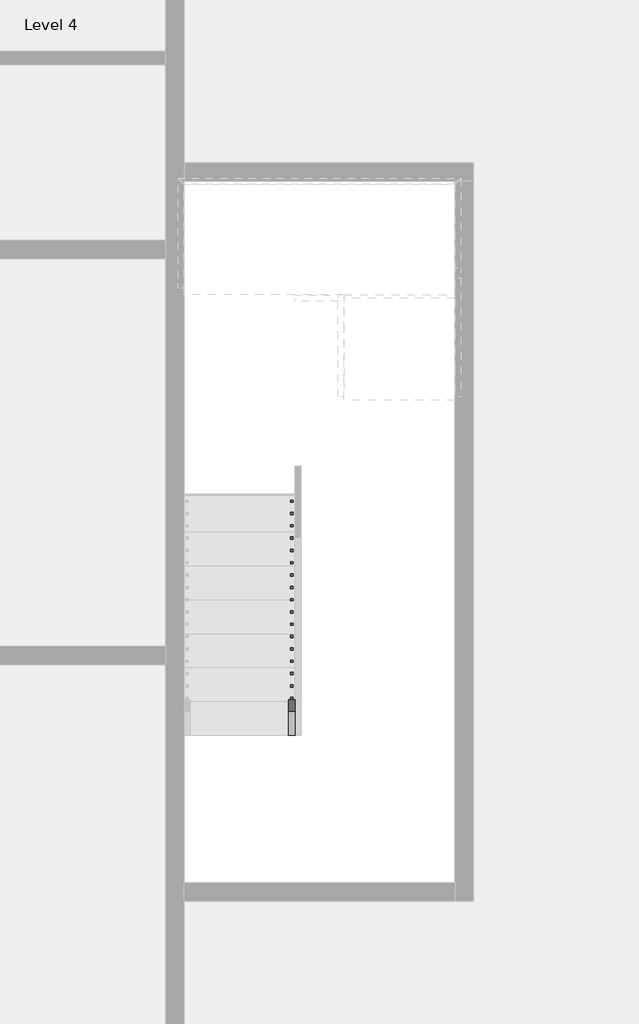
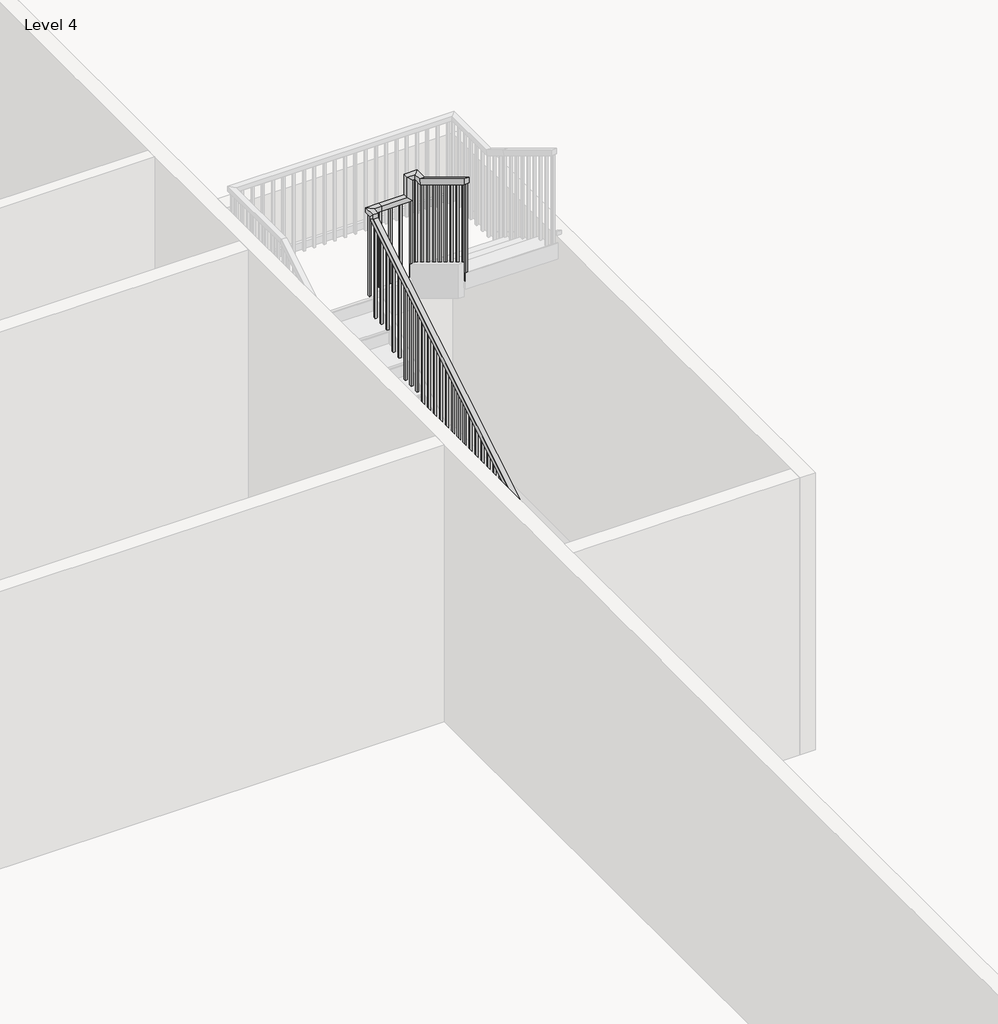
# One storey, part 5 of 8: 1 railing.
"""IFC4 building model written with IfcOpenShell, lengths in millimetres."""

from ifc_helpers import new_model, si_unit, frame, origin, place, context, project, spatial, polyline, outline, extrude, faceted_brep, element, save

model = new_model("IFC4")

# Units and contexts
model_context = context("Model", 3, world=origin())
ifc_project = project(units=[si_unit("LENGTHUNIT", "METRE", prefix="MILLI")], contexts=[model_context])

# Site, building, storey
site = spatial("IfcSite", under=ifc_project)
building = spatial("IfcBuilding", under=site)
storey = spatial("IfcBuildingStorey", under=building, Name="Level 4", Elevation=34378.6172466)

# Railing
placement = place(None, origin())
element("IfcRailing", 1, ObjectType="Handrail - Rectangular", at=placement, inside=storey, context=model_context, shape_type="SolidModel", body=[
    faceted_brep([(-2753.8415084, -23154.3851539, 35462.3505799), (-2753.8415084, -23154.3851539, 35402.9491197), (-2703.0415084, -23154.3851539, 35402.9491197), (-2703.0415084, -23154.3851539, 35462.3505799), (-2753.8415084, -19598.3851539, 37617.5020951), (-2753.8415084, -19547.5851539, 37588.8885136), (-2703.0415084, -19547.5851539, 37588.8885136), (-2703.0415084, -19598.3851539, 37617.5020951), (-2753.8415084, -19598.3851539, 37663.6839133), (-2753.8415084, -19547.5851539, 37612.8839133), (-2703.0415084, -19547.5851539, 37612.8839133), (-2703.0415084, -19598.3851539, 37663.6839133), (-2753.8415084, -19471.3851539, 37663.6839133), (-2753.8415084, -19471.3851539, 37612.8839133), (-2703.0415084, -19522.1851539, 37612.8839133), (-2703.0415084, -19522.1851539, 37663.6839133), (-2626.8415084, -19471.3851539, 37663.6839133), (-2626.8415084, -19471.3851539, 37612.8839133), (-2626.8415084, -19522.1851539, 37612.8839133), (-2626.8415084, -19522.1851539, 37663.6839133), (-2372.8415084, -19471.3851539, 37663.6839133), (-2322.0415084, -19471.3851539, 37612.8839133), (-2322.0415084, -19522.1851539, 37612.8839133), (-2372.8415084, -19522.1851539, 37663.6839133), (-2372.8415084, -19471.3851539, 37879.1990648), (-2322.0415084, -19471.3851539, 37828.3990648), (-2322.0415084, -19522.1851539, 37828.3990648), (-2372.8415084, -19522.1851539, 37879.1990648), (-2245.8415084, -19471.3851539, 37879.1990648), (-2245.8415084, -19471.3851539, 37828.3990648), (-2296.6415084, -19522.1851539, 37828.3990648), (-2296.6415084, -19522.1851539, 37879.1990648), (-2245.8415084, -19598.3851539, 37879.1990648), (-2245.8415084, -19612.5775633, 37828.3990648), (-2296.6415084, -19612.5775633, 37828.3990648), (-2296.6415084, -19598.3851539, 37879.1990648), (-2245.8415084, -20360.3851539, 38341.0172466), (-2296.6415084, -20360.3851539, 38341.0172466), (-2296.6415084, -20360.3851539, 38281.6157863), (-2245.8415084, -20360.3851539, 38281.6157863)], [[[0, 1, 2, 3]], [[1, 0, 4, 5]], [[2, 1, 5, 6]], [[3, 2, 6, 7]], [[0, 3, 7, 4]], [[5, 4, 8, 9]], [[6, 5, 9, 10]], [[7, 6, 10, 11]], [[4, 7, 11, 8]], [[9, 8, 12, 13]], [[10, 9, 13, 14]], [[11, 10, 14, 15]], [[8, 11, 15, 12]], [[13, 12, 16, 17]], [[14, 13, 17, 18]], [[15, 14, 18, 19]], [[12, 15, 19, 16]], [[17, 16, 20, 21]], [[18, 17, 21, 22]], [[19, 18, 22, 23]], [[16, 19, 23, 20]], [[21, 20, 24, 25]], [[22, 21, 25, 26]], [[23, 22, 26, 27]], [[20, 23, 27, 24]], [[25, 24, 28, 29]], [[26, 25, 29, 30]], [[27, 26, 30, 31]], [[24, 27, 31, 28]], [[29, 28, 32, 33]], [[30, 29, 33, 34]], [[31, 30, 34, 35]], [[28, 31, 35, 32]], [[36, 37, 38, 39]], [[33, 32, 36, 39]], [[34, 33, 39, 38]], [[35, 34, 38, 37]], [[32, 35, 37, 36]]]),
    extrude(outline(polyline([(-20319.1101539, 38256.6006348), (-20300.0601539, 38245.0551803), (-20300.0601539, 37257.2839133), (-20319.1101539, 37257.2839133), (-20319.1101539, 38256.6006348)])), frame((-2280.7665084, 0.0, 0.0), z_axis=(1.0, 0.0, 0.0), x_axis=(0.0, 1.0, 0.0)), (0.0, 0.0, 1.0), 19.05),
    extrude(outline(polyline([(-20217.5101539, 38195.0248773), (-20198.4601539, 38183.4794227), (-20198.4601539, 37257.2839133), (-20217.5101539, 37257.2839133), (-20217.5101539, 38195.0248773)])), frame((-2280.7665084, 0.0, 0.0), z_axis=(1.0, 0.0, 0.0), x_axis=(0.0, 1.0, 0.0)), (0.0, 0.0, 1.0), 19.05),
    extrude(outline(polyline([(-20115.9101539, 38133.4491197), (-20096.8601539, 38121.9036651), (-20096.8601539, 37257.2839133), (-20115.9101539, 37257.2839133), (-20115.9101539, 38133.4491197)])), frame((-2280.7665084, 0.0, 0.0), z_axis=(1.0, 0.0, 0.0), x_axis=(0.0, 1.0, 0.0)), (0.0, 0.0, 1.0), 19.05),
    extrude(outline(polyline([(-20014.3101539, 38071.8733621), (-19995.2601539, 38060.3279076), (-19995.2601539, 37087.9505799), (-20014.3101539, 37087.9505799), (-20014.3101539, 38071.8733621)])), frame((-2280.7665084, 0.0, 0.0), z_axis=(1.0, 0.0, 0.0), x_axis=(0.0, 1.0, 0.0)), (0.0, 0.0, 1.0), 19.05),
    extrude(outline(polyline([(-19912.7101539, 38010.2976045), (-19893.6601539, 37998.75215), (-19893.6601539, 37087.9505799), (-19912.7101539, 37087.9505799), (-19912.7101539, 38010.2976045)])), frame((-2280.7665084, 0.0, 0.0), z_axis=(1.0, 0.0, 0.0), x_axis=(0.0, 1.0, 0.0)), (0.0, 0.0, 1.0), 19.05),
    extrude(outline(polyline([(-19811.1101539, 37948.721847), (-19792.0601539, 37937.1763924), (-19792.0601539, 37087.9505799), (-19811.1101539, 37087.9505799), (-19811.1101539, 37948.721847)])), frame((-2280.7665084, 0.0, 0.0), z_axis=(1.0, 0.0, 0.0), x_axis=(0.0, 1.0, 0.0)), (0.0, 0.0, 1.0), 19.05),
    extrude(outline(polyline([(-19709.5101539, 37887.1460894), (-19690.4601539, 37875.6006348), (-19690.4601539, 36918.6172466), (-19709.5101539, 36918.6172466), (-19709.5101539, 37887.1460894)])), frame((-2280.7665084, 0.0, 0.0), z_axis=(1.0, 0.0, 0.0), x_axis=(0.0, 1.0, 0.0)), (0.0, 0.0, 1.0), 19.05),
    extrude(outline(polyline([(-19607.9101539, 37825.5703318), (-19588.8601539, 37814.0248773), (-19588.8601539, 36918.6172466), (-19607.9101539, 36918.6172466), (-19607.9101539, 37825.5703318)])), frame((-2280.7665084, 0.0, 0.0), z_axis=(1.0, 0.0, 0.0), x_axis=(0.0, 1.0, 0.0)), (0.0, 0.0, 1.0), 19.05),
    extrude(outline(polyline([(-2331.5665084, -19506.3101539), (-2331.5665084, -19487.2601539), (-2312.5165084, -19487.2601539), (-2312.5165084, -19506.3101539), (-2331.5665084, -19506.3101539)])), frame((0.0, 0.0, 36749.2839133), z_axis=(0.0, 0.0, 1.0), x_axis=(1.0, 0.0, 0.0)), (0.0, 0.0, 1.0), 1079.1151515),
    extrude(outline(polyline([(-2433.1665084, -19506.3101539), (-2433.1665084, -19487.2601539), (-2414.1165084, -19487.2601539), (-2414.1165084, -19506.3101539), (-2433.1665084, -19506.3101539)])), frame((0.0, 0.0, 36749.2839133), z_axis=(0.0, 0.0, 1.0), x_axis=(1.0, 0.0, 0.0)), (0.0, 0.0, 1.0), 863.6),
    extrude(outline(polyline([(-2534.7665084, -19506.3101539), (-2534.7665084, -19487.2601539), (-2515.7165084, -19487.2601539), (-2515.7165084, -19506.3101539), (-2534.7665084, -19506.3101539)])), frame((0.0, 0.0, 36749.2839133), z_axis=(0.0, 0.0, 1.0), x_axis=(1.0, 0.0, 0.0)), (0.0, 0.0, 1.0), 863.6),
    extrude(outline(polyline([(-2636.3665084, -19506.3101539), (-2636.3665084, -19487.2601539), (-2617.3165084, -19487.2601539), (-2617.3165084, -19506.3101539), (-2636.3665084, -19506.3101539)])), frame((0.0, 0.0, 36749.2839133), z_axis=(0.0, 0.0, 1.0), x_axis=(1.0, 0.0, 0.0)), (0.0, 0.0, 1.0), 863.6),
    extrude(outline(polyline([(-19607.9101539, 37552.3279076), (-19588.8601539, 37563.8733621), (-19588.8601539, 36579.9505799), (-19607.9101539, 36579.9505799), (-19607.9101539, 37552.3279076)])), frame((-2737.9665084, 0.0, 0.0), z_axis=(1.0, 0.0, 0.0), x_axis=(0.0, 1.0, 0.0)), (0.0, 0.0, 1.0), 19.05),
    extrude(outline(polyline([(-19709.5101539, 37490.75215), (-19690.4601539, 37502.2976045), (-19690.4601539, 36579.9505799), (-19709.5101539, 36579.9505799), (-19709.5101539, 37490.75215)])), frame((-2737.9665084, 0.0, 0.0), z_axis=(1.0, 0.0, 0.0), x_axis=(0.0, 1.0, 0.0)), (0.0, 0.0, 1.0), 19.05),
    extrude(outline(polyline([(-19811.1101539, 37429.1763924), (-19792.0601539, 37440.721847), (-19792.0601539, 36579.9505799), (-19811.1101539, 36579.9505799), (-19811.1101539, 37429.1763924)])), frame((-2737.9665084, 0.0, 0.0), z_axis=(1.0, 0.0, 0.0), x_axis=(0.0, 1.0, 0.0)), (0.0, 0.0, 1.0), 19.05),
    extrude(outline(polyline([(-19912.7101539, 37367.6006348), (-19893.6601539, 37379.1460894), (-19893.6601539, 36410.6172466), (-19912.7101539, 36410.6172466), (-19912.7101539, 37367.6006348)])), frame((-2737.9665084, 0.0, 0.0), z_axis=(1.0, 0.0, 0.0), x_axis=(0.0, 1.0, 0.0)), (0.0, 0.0, 1.0), 19.05),
    extrude(outline(polyline([(-20014.3101539, 37306.0248773), (-19995.2601539, 37317.5703318), (-19995.2601539, 36410.6172466), (-20014.3101539, 36410.6172466), (-20014.3101539, 37306.0248773)])), frame((-2737.9665084, 0.0, 0.0), z_axis=(1.0, 0.0, 0.0), x_axis=(0.0, 1.0, 0.0)), (0.0, 0.0, 1.0), 19.05),
    extrude(outline(polyline([(-20115.9101539, 37244.4491197), (-20096.8601539, 37255.9945742), (-20096.8601539, 36241.2839133), (-20115.9101539, 36241.2839133), (-20115.9101539, 37244.4491197)])), frame((-2737.9665084, 0.0, 0.0), z_axis=(1.0, 0.0, 0.0), x_axis=(0.0, 1.0, 0.0)), (0.0, 0.0, 1.0), 19.05),
    extrude(outline(polyline([(-20217.5101539, 37182.8733621), (-20198.4601539, 37194.4188166), (-20198.4601539, 36241.2839133), (-20217.5101539, 36241.2839133), (-20217.5101539, 37182.8733621)])), frame((-2737.9665084, 0.0, 0.0), z_axis=(1.0, 0.0, 0.0), x_axis=(0.0, 1.0, 0.0)), (0.0, 0.0, 1.0), 19.05),
    extrude(outline(polyline([(-20319.1101539, 37121.2976045), (-20300.0601539, 37132.8430591), (-20300.0601539, 36241.2839133), (-20319.1101539, 36241.2839133), (-20319.1101539, 37121.2976045)])), frame((-2737.9665084, 0.0, 0.0), z_axis=(1.0, 0.0, 0.0), x_axis=(0.0, 1.0, 0.0)), (0.0, 0.0, 1.0), 19.05),
    extrude(outline(polyline([(-20420.7101539, 37059.721847), (-20401.6601539, 37071.2673015), (-20401.6601539, 36071.9505799), (-20420.7101539, 36071.9505799), (-20420.7101539, 37059.721847)])), frame((-2737.9665084, 0.0, 0.0), z_axis=(1.0, 0.0, 0.0), x_axis=(0.0, 1.0, 0.0)), (0.0, 0.0, 1.0), 19.05),
    extrude(outline(polyline([(-20522.3101539, 36998.1460894), (-20503.2601539, 37009.6915439), (-20503.2601539, 36071.9505799), (-20522.3101539, 36071.9505799), (-20522.3101539, 36998.1460894)])), frame((-2737.9665084, 0.0, 0.0), z_axis=(1.0, 0.0, 0.0), x_axis=(0.0, 1.0, 0.0)), (0.0, 0.0, 1.0), 19.05),
    extrude(outline(polyline([(-20623.9101539, 36936.5703318), (-20604.8601539, 36948.1157863), (-20604.8601539, 36071.9505799), (-20623.9101539, 36071.9505799), (-20623.9101539, 36936.5703318)])), frame((-2737.9665084, 0.0, 0.0), z_axis=(1.0, 0.0, 0.0), x_axis=(0.0, 1.0, 0.0)), (0.0, 0.0, 1.0), 19.05),
    extrude(outline(polyline([(-20725.5101539, 36874.9945742), (-20706.4601539, 36886.5400288), (-20706.4601539, 35902.6172466), (-20725.5101539, 35902.6172466), (-20725.5101539, 36874.9945742)])), frame((-2737.9665084, 0.0, 0.0), z_axis=(1.0, 0.0, 0.0), x_axis=(0.0, 1.0, 0.0)), (0.0, 0.0, 1.0), 19.05),
    extrude(outline(polyline([(-20827.1101539, 36813.4188166), (-20808.0601539, 36824.9642712), (-20808.0601539, 35902.6172466), (-20827.1101539, 35902.6172466), (-20827.1101539, 36813.4188166)])), frame((-2737.9665084, 0.0, 0.0), z_axis=(1.0, 0.0, 0.0), x_axis=(0.0, 1.0, 0.0)), (0.0, 0.0, 1.0), 19.05),
    extrude(outline(polyline([(-20928.7101539, 36751.8430591), (-20909.6601539, 36763.3885136), (-20909.6601539, 35902.6172466), (-20928.7101539, 35902.6172466), (-20928.7101539, 36751.8430591)])), frame((-2737.9665084, 0.0, 0.0), z_axis=(1.0, 0.0, 0.0), x_axis=(0.0, 1.0, 0.0)), (0.0, 0.0, 1.0), 19.05),
    extrude(outline(polyline([(-21030.3101539, 36690.2673015), (-21011.2601539, 36701.812756), (-21011.2601539, 35733.2839133), (-21030.3101539, 35733.2839133), (-21030.3101539, 36690.2673015)])), frame((-2737.9665084, 0.0, 0.0), z_axis=(1.0, 0.0, 0.0), x_axis=(0.0, 1.0, 0.0)), (0.0, 0.0, 1.0), 19.05),
    extrude(outline(polyline([(-21131.9101539, 36628.6915439), (-21112.8601539, 36640.2369985), (-21112.8601539, 35733.2839133), (-21131.9101539, 35733.2839133), (-21131.9101539, 36628.6915439)])), frame((-2737.9665084, 0.0, 0.0), z_axis=(1.0, 0.0, 0.0), x_axis=(0.0, 1.0, 0.0)), (0.0, 0.0, 1.0), 19.05),
    extrude(outline(polyline([(-21233.5101539, 36567.1157863), (-21214.4601539, 36578.6612409), (-21214.4601539, 35563.9505799), (-21233.5101539, 35563.9505799), (-21233.5101539, 36567.1157863)])), frame((-2737.9665084, 0.0, 0.0), z_axis=(1.0, 0.0, 0.0), x_axis=(0.0, 1.0, 0.0)), (0.0, 0.0, 1.0), 19.05),
    extrude(outline(polyline([(-21335.1101539, 36505.5400288), (-21316.0601539, 36517.0854833), (-21316.0601539, 35563.9505799), (-21335.1101539, 35563.9505799), (-21335.1101539, 36505.5400288)])), frame((-2737.9665084, 0.0, 0.0), z_axis=(1.0, 0.0, 0.0), x_axis=(0.0, 1.0, 0.0)), (0.0, 0.0, 1.0), 19.05),
    extrude(outline(polyline([(-21436.7101539, 36443.9642712), (-21417.6601539, 36455.5097257), (-21417.6601539, 35563.9505799), (-21436.7101539, 35563.9505799), (-21436.7101539, 36443.9642712)])), frame((-2737.9665084, 0.0, 0.0), z_axis=(1.0, 0.0, 0.0), x_axis=(0.0, 1.0, 0.0)), (0.0, 0.0, 1.0), 19.05),
    extrude(outline(polyline([(-21538.3101539, 36382.3885136), (-21519.2601539, 36393.9339682), (-21519.2601539, 35394.6172466), (-21538.3101539, 35394.6172466), (-21538.3101539, 36382.3885136)])), frame((-2737.9665084, 0.0, 0.0), z_axis=(1.0, 0.0, 0.0), x_axis=(0.0, 1.0, 0.0)), (0.0, 0.0, 1.0), 19.05),
    extrude(outline(polyline([(-21639.9101539, 36320.812756), (-21620.8601539, 36332.3582106), (-21620.8601539, 35394.6172466), (-21639.9101539, 35394.6172466), (-21639.9101539, 36320.812756)])), frame((-2737.9665084, 0.0, 0.0), z_axis=(1.0, 0.0, 0.0), x_axis=(0.0, 1.0, 0.0)), (0.0, 0.0, 1.0), 19.05),
    extrude(outline(polyline([(-21741.5101539, 36259.2369985), (-21722.4601539, 36270.782453), (-21722.4601539, 35394.6172466), (-21741.5101539, 35394.6172466), (-21741.5101539, 36259.2369985)])), frame((-2737.9665084, 0.0, 0.0), z_axis=(1.0, 0.0, 0.0), x_axis=(0.0, 1.0, 0.0)), (0.0, 0.0, 1.0), 19.05),
    extrude(outline(polyline([(-21843.1101539, 36197.6612409), (-21824.0601539, 36209.2066954), (-21824.0601539, 35225.2839133), (-21843.1101539, 35225.2839133), (-21843.1101539, 36197.6612409)])), frame((-2737.9665084, 0.0, 0.0), z_axis=(1.0, 0.0, 0.0), x_axis=(0.0, 1.0, 0.0)), (0.0, 0.0, 1.0), 19.05),
    extrude(outline(polyline([(-21944.7101539, 36136.0854833), (-21925.6601539, 36147.6309379), (-21925.6601539, 35225.2839133), (-21944.7101539, 35225.2839133), (-21944.7101539, 36136.0854833)])), frame((-2737.9665084, 0.0, 0.0), z_axis=(1.0, 0.0, 0.0), x_axis=(0.0, 1.0, 0.0)), (0.0, 0.0, 1.0), 19.05),
    extrude(outline(polyline([(-22046.3101539, 36074.5097257), (-22027.2601539, 36086.0551803), (-22027.2601539, 35225.2839133), (-22046.3101539, 35225.2839133), (-22046.3101539, 36074.5097257)])), frame((-2737.9665084, 0.0, 0.0), z_axis=(1.0, 0.0, 0.0), x_axis=(0.0, 1.0, 0.0)), (0.0, 0.0, 1.0), 19.05),
    extrude(outline(polyline([(-22147.9101539, 36012.9339682), (-22128.8601539, 36024.4794227), (-22128.8601539, 35055.9505799), (-22147.9101539, 35055.9505799), (-22147.9101539, 36012.9339682)])), frame((-2737.9665084, 0.0, 0.0), z_axis=(1.0, 0.0, 0.0), x_axis=(0.0, 1.0, 0.0)), (0.0, 0.0, 1.0), 19.05),
    extrude(outline(polyline([(-22249.5101539, 35951.3582106), (-22230.4601539, 35962.9036651), (-22230.4601539, 35055.9505799), (-22249.5101539, 35055.9505799), (-22249.5101539, 35951.3582106)])), frame((-2737.9665084, 0.0, 0.0), z_axis=(1.0, 0.0, 0.0), x_axis=(0.0, 1.0, 0.0)), (0.0, 0.0, 1.0), 19.05),
    extrude(outline(polyline([(-22351.1101539, 35889.782453), (-22332.0601539, 35901.3279076), (-22332.0601539, 34886.6172466), (-22351.1101539, 34886.6172466), (-22351.1101539, 35889.782453)])), frame((-2737.9665084, 0.0, 0.0), z_axis=(1.0, 0.0, 0.0), x_axis=(0.0, 1.0, 0.0)), (0.0, 0.0, 1.0), 19.05),
    extrude(outline(polyline([(-22452.7101539, 35828.2066954), (-22433.6601539, 35839.75215), (-22433.6601539, 34886.6172466), (-22452.7101539, 34886.6172466), (-22452.7101539, 35828.2066954)])), frame((-2737.9665084, 0.0, 0.0), z_axis=(1.0, 0.0, 0.0), x_axis=(0.0, 1.0, 0.0)), (0.0, 0.0, 1.0), 19.05),
    extrude(outline(polyline([(-22554.3101539, 35766.6309379), (-22535.2601539, 35778.1763924), (-22535.2601539, 34886.6172466), (-22554.3101539, 34886.6172466), (-22554.3101539, 35766.6309379)])), frame((-2737.9665084, 0.0, 0.0), z_axis=(1.0, 0.0, 0.0), x_axis=(0.0, 1.0, 0.0)), (0.0, 0.0, 1.0), 19.05),
    extrude(outline(polyline([(-22655.9101539, 35705.0551803), (-22636.8601539, 35716.6006348), (-22636.8601539, 34717.2839133), (-22655.9101539, 34717.2839133), (-22655.9101539, 35705.0551803)])), frame((-2737.9665084, 0.0, 0.0), z_axis=(1.0, 0.0, 0.0), x_axis=(0.0, 1.0, 0.0)), (0.0, 0.0, 1.0), 19.05),
    extrude(outline(polyline([(-22757.5101539, 35643.4794227), (-22738.4601539, 35655.0248773), (-22738.4601539, 34717.2839133), (-22757.5101539, 34717.2839133), (-22757.5101539, 35643.4794227)])), frame((-2737.9665084, 0.0, 0.0), z_axis=(1.0, 0.0, 0.0), x_axis=(0.0, 1.0, 0.0)), (0.0, 0.0, 1.0), 19.05),
    extrude(outline(polyline([(-22859.1101539, 35581.9036651), (-22840.0601539, 35593.4491197), (-22840.0601539, 34717.2839133), (-22859.1101539, 34717.2839133), (-22859.1101539, 35581.9036651)])), frame((-2737.9665084, 0.0, 0.0), z_axis=(1.0, 0.0, 0.0), x_axis=(0.0, 1.0, 0.0)), (0.0, 0.0, 1.0), 19.05),
    extrude(outline(polyline([(-22960.7101539, 35520.3279076), (-22941.6601539, 35531.8733621), (-22941.6601539, 34547.9505799), (-22960.7101539, 34547.9505799), (-22960.7101539, 35520.3279076)])), frame((-2737.9665084, 0.0, 0.0), z_axis=(1.0, 0.0, 0.0), x_axis=(0.0, 1.0, 0.0)), (0.0, 0.0, 1.0), 19.05),
    extrude(outline(polyline([(-23062.3101539, 35458.75215), (-23043.2601539, 35470.2976045), (-23043.2601539, 34547.9505799), (-23062.3101539, 34547.9505799), (-23062.3101539, 35458.75215)])), frame((-2737.9665084, 0.0, 0.0), z_axis=(1.0, 0.0, 0.0), x_axis=(0.0, 1.0, 0.0)), (0.0, 0.0, 1.0), 19.05),
    extrude(outline(polyline([(-2280.7665084, -19506.3101539), (-2280.7665084, -19487.2601539), (-2261.7165084, -19487.2601539), (-2261.7165084, -19506.3101539), (-2280.7665084, -19506.3101539)])), frame((0.0, 0.0, 36749.2839133), z_axis=(0.0, 0.0, 1.0), x_axis=(1.0, 0.0, 0.0)), (0.0, 0.0, 1.0), 1079.1151515),
    extrude(outline(polyline([(-2718.9165084, -19506.3101539), (-2737.9665084, -19506.3101539), (-2737.9665084, -19487.2601539), (-2718.9165084, -19487.2601539), (-2718.9165084, -19506.3101539)])), frame((0.0, 0.0, 36749.2839133), z_axis=(0.0, 0.0, 1.0), x_axis=(1.0, 0.0, 0.0)), (0.0, 0.0, 1.0), 863.6),
    extrude(outline(polyline([(-20360.3851539, 38281.6157863), (-20341.3351539, 38270.0703318), (-20341.3351539, 37257.2839133), (-20360.3851539, 37257.2839133), (-20360.3851539, 38281.6157863)])), frame((-2280.7665084, 0.0, 0.0), z_axis=(1.0, 0.0, 0.0), x_axis=(0.0, 1.0, 0.0)), (0.0, 0.0, 1.0), 19.05),
    extrude(outline(polyline([(-23154.3851539, 35402.9491197), (-23135.3351539, 35414.4945742), (-23135.3351539, 34547.9505799), (-23154.3851539, 34547.9505799), (-23154.3851539, 35402.9491197)])), frame((-2737.9665084, 0.0, 0.0), z_axis=(1.0, 0.0, 0.0), x_axis=(0.0, 1.0, 0.0)), (0.0, 0.0, 1.0), 19.05),
])

save(model, "model.ifc")

# Revit data of these elements
# Type "Handrail - Rectangular"
#   Assembly Code = "C2010400"
#   built-in parameter 1008612 = 0.0416667 (stored number, unit not read)
#   built-in parameter 1008611 = 0.0416667 (stored number, unit not read)
#   built-in parameter 1008609 = 0.333333 (stored number, unit not read)
#   built-in parameter 1008604 = 0.166667 (stored number, unit not read)
#   built-in parameter 1008603 = 0.166667 (stored number, unit not read)
#   Railing Height = 3' - 0"
#   built-in parameter 1008630 = 2
#   built-in parameter 1008610 = 2
#   built-in parameter 1008618 = Baluster - Square : 3/4"
# Element 1 (IfcRailing, "Handrail - Rectangular")
#   Phase Created = New Construction
